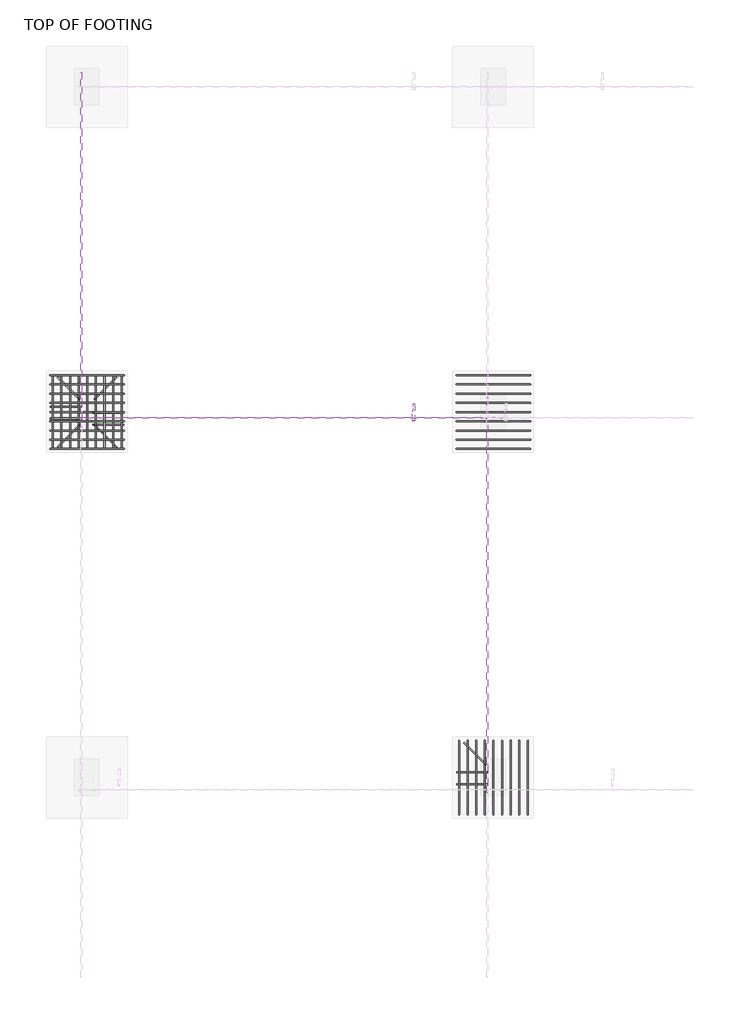
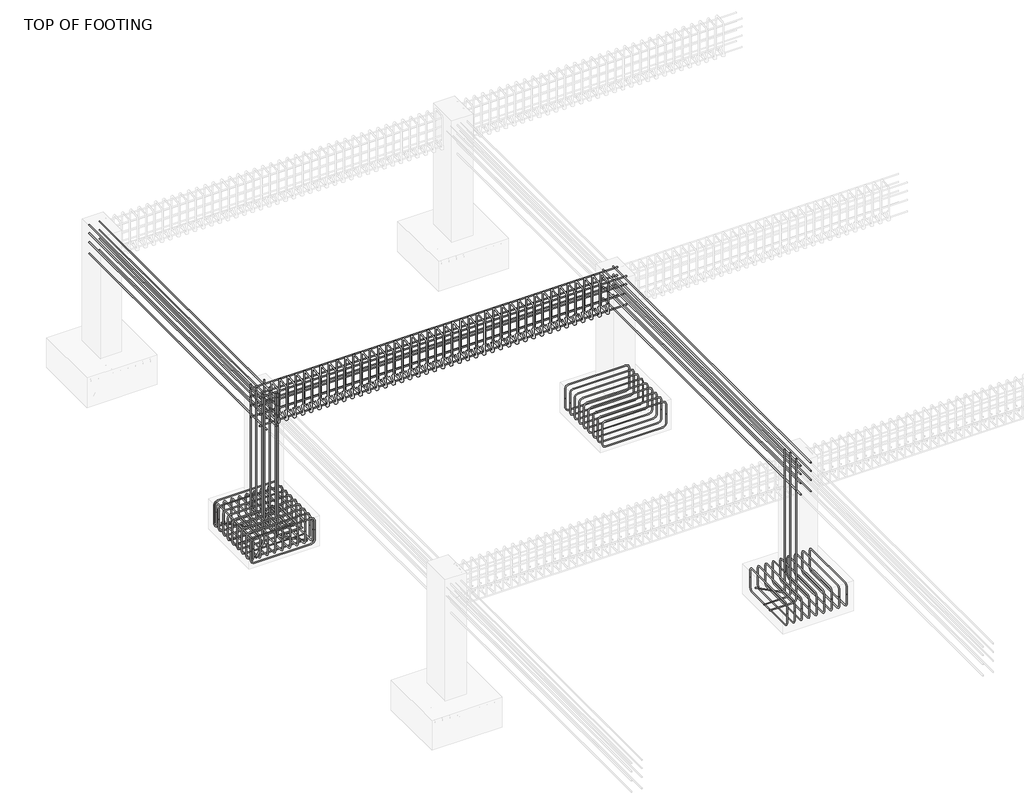
# One storey, part 5 of 13: 29 reinforcing bars.
"""IFC4 building model written with IfcOpenShell, lengths in millimetres."""

from ifc_helpers import new_model, si_unit, point, frame, origin, place, context, project, spatial, polyline, circle_curve, trimmed, segment, composite_curve, source, transform, mapped, element, save
from ifc_brep_helpers import swept_disk

model = new_model("IFC4")

# Units and contexts
model_context = context("Model", 3, world=origin())
ifc_project = project(units=[si_unit("LENGTHUNIT", "METRE", prefix="MILLI")], contexts=[model_context])

# Site, building, storey
site = spatial("IfcSite", under=ifc_project)
building = spatial("IfcBuilding", under=site)
storey = spatial("IfcBuildingStorey", under=building, Name="TOP OF FOOTING", Elevation=-1828.8)

# Reinforcing bars
placement = place(None, origin())
reinforcing_bar_shape = source(origin(), model_context, "Body", "SolidModel", [
    swept_disk(composite_curve([segment(polyline([(-12666.6498378, 12986.1851908, -2049.322685), (-12666.6498378, 12986.1851908, -2196.622685)]), True, "CONTINUOUS"), segment(trimmed(circle_curve(frame((-12712.9998378, 12986.1851908, -2196.622685), z_axis=(0.0, 1.0, 0.0), x_axis=(46.350000000000364, 0.0, 0.0)), 46.35), [point((-12666.6498378, 12986.1851908, -2196.622685))], [point((-12712.9998378, 12986.1851908, -2242.972685))], True, "CARTESIAN"), True, "CONTINUOUS"), segment(polyline([(-12712.9998378, 12986.1851908, -2242.972685), (-13527.5998378, 12986.1851908, -2242.972685)]), True, "CONTINUOUS"), segment(trimmed(circle_curve(frame((-13527.5998378, 12986.1851908, -2196.622685), z_axis=(0.0, 1.0, 0.0), x_axis=(0.0, 0.0, -46.350000000000364)), 46.35), [point((-13527.5998378, 12986.1851908, -2242.972685))], [point((-13573.9498378, 12986.1851908, -2196.622685))], True, "CARTESIAN"), True, "CONTINUOUS"), segment(polyline([(-13573.9498378, 12986.1851908, -2196.622685), (-13573.9498378, 12986.1851908, -2049.322685)]), True, "CONTINUOUS")], self_intersect=False), 6.35),
])
element("IfcReinforcingBar", 1, at=placement, inside=storey, context=model_context, shape_type="MappedRepresentation", body=[
    mapped(reinforcing_bar_shape, transform((0.0, 0.0, 0.0), x_axis=(1.0, 0.0, 0.0), y_axis=(0.0, 1.0, 0.0), z_axis=(0.0, 0.0, 1.0))),
    mapped(reinforcing_bar_shape, transform((0.0, -113.4125, 0.0), x_axis=(1.0, 0.0, 0.0), y_axis=(0.0, 1.0, 0.0), z_axis=(0.0, 0.0, 1.0))),
    mapped(reinforcing_bar_shape, transform((0.0, -226.825, 0.0), x_axis=(1.0, 0.0, 0.0), y_axis=(0.0, 1.0, 0.0), z_axis=(0.0, 0.0, 1.0))),
    mapped(reinforcing_bar_shape, transform((0.0, -340.2375, 0.0), x_axis=(1.0, 0.0, 0.0), y_axis=(0.0, 1.0, 0.0), z_axis=(0.0, 0.0, 1.0))),
    mapped(reinforcing_bar_shape, transform((0.0, -453.65, 0.0), x_axis=(1.0, 0.0, 0.0), y_axis=(0.0, 1.0, 0.0), z_axis=(0.0, 0.0, 1.0))),
    mapped(reinforcing_bar_shape, transform((0.0, -567.0625, 0.0), x_axis=(1.0, 0.0, 0.0), y_axis=(0.0, 1.0, 0.0), z_axis=(0.0, 0.0, 1.0))),
    mapped(reinforcing_bar_shape, transform((0.0, -680.475, 0.0), x_axis=(1.0, 0.0, 0.0), y_axis=(0.0, 1.0, 0.0), z_axis=(0.0, 0.0, 1.0))),
    mapped(reinforcing_bar_shape, transform((0.0, -793.8875, 0.0), x_axis=(1.0, 0.0, 0.0), y_axis=(0.0, 1.0, 0.0), z_axis=(0.0, 0.0, 1.0))),
    mapped(reinforcing_bar_shape, transform((0.0, -907.3, 0.0), x_axis=(1.0, 0.0, 0.0), y_axis=(0.0, 1.0, 0.0), z_axis=(0.0, 0.0, 1.0))),
])
reinforcing_bar_2_shape = source(origin(), model_context, "Body", "SolidModel", [
    swept_disk(composite_curve([segment(polyline([(-13573.9498378, 12986.1851908, -2051.3998363), (-13573.9498378, 12986.1851908, -1904.0998363)]), True, "CONTINUOUS"), segment(trimmed(circle_curve(frame((-13527.5998378, 12986.1851908, -1904.0998363), z_axis=(0.0, 1.0, 0.0), x_axis=(-46.350000000000364, 0.0, 0.0)), 46.35), [point((-13573.9498378, 12986.1851908, -1904.0998363))], [point((-13527.5998378, 12986.1851908, -1857.7498363))], True, "CARTESIAN"), True, "CONTINUOUS"), segment(polyline([(-13527.5998378, 12986.1851908, -1857.7498363), (-12712.9998378, 12986.1851908, -1857.7498363)]), True, "CONTINUOUS"), segment(trimmed(circle_curve(frame((-12712.9998378, 12986.1851908, -1904.0998363), z_axis=(0.0, 1.0, 0.0), x_axis=(0.0, 0.0, 46.350000000000136)), 46.35), [point((-12712.9998378, 12986.1851908, -1857.7498363))], [point((-12666.6498378, 12986.1851908, -1904.0998363))], True, "CARTESIAN"), True, "CONTINUOUS"), segment(polyline([(-12666.6498378, 12986.1851908, -1904.0998363), (-12666.6498378, 12986.1851908, -2051.3998363)]), True, "CONTINUOUS")], self_intersect=False), 6.35),
])
element("IfcReinforcingBar", 2, at=placement, inside=storey, context=model_context, shape_type="MappedRepresentation", body=[
    mapped(reinforcing_bar_2_shape, transform((0.0, 0.0, 0.0), x_axis=(1.0, 0.0, 0.0), y_axis=(0.0, 1.0, 0.0), z_axis=(0.0, 0.0, 1.0))),
    mapped(reinforcing_bar_2_shape, transform((0.0, -113.4125, 0.0), x_axis=(1.0, 0.0, 0.0), y_axis=(0.0, 1.0, 0.0), z_axis=(0.0, 0.0, 1.0))),
    mapped(reinforcing_bar_2_shape, transform((0.0, -226.825, 0.0), x_axis=(1.0, 0.0, 0.0), y_axis=(0.0, 1.0, 0.0), z_axis=(0.0, 0.0, 1.0))),
    mapped(reinforcing_bar_2_shape, transform((0.0, -340.2375, 0.0), x_axis=(1.0, 0.0, 0.0), y_axis=(0.0, 1.0, 0.0), z_axis=(0.0, 0.0, 1.0))),
    mapped(reinforcing_bar_2_shape, transform((0.0, -453.65, 0.0), x_axis=(1.0, 0.0, 0.0), y_axis=(0.0, 1.0, 0.0), z_axis=(0.0, 0.0, 1.0))),
    mapped(reinforcing_bar_2_shape, transform((0.0, -567.0625, 0.0), x_axis=(1.0, 0.0, 0.0), y_axis=(0.0, 1.0, 0.0), z_axis=(0.0, 0.0, 1.0))),
    mapped(reinforcing_bar_2_shape, transform((0.0, -680.475, 0.0), x_axis=(1.0, 0.0, 0.0), y_axis=(0.0, 1.0, 0.0), z_axis=(0.0, 0.0, 1.0))),
    mapped(reinforcing_bar_2_shape, transform((0.0, -793.8875, 0.0), x_axis=(1.0, 0.0, 0.0), y_axis=(0.0, 1.0, 0.0), z_axis=(0.0, 0.0, 1.0))),
    mapped(reinforcing_bar_2_shape, transform((0.0, -907.3, 0.0), x_axis=(1.0, 0.0, 0.0), y_axis=(0.0, 1.0, 0.0), z_axis=(0.0, 0.0, 1.0))),
])
reinforcing_bar_3_shape = source(origin(), model_context, "Body", "SolidModel", [
    swept_disk(composite_curve([segment(polyline([(-13542.4641345, 12986.1851908, -2025.081839), (-13542.4641345, 12986.1851908, -2172.381839)]), True, "CONTINUOUS"), segment(trimmed(circle_curve(frame((-13542.4641345, 12939.8351908, -2172.381839), z_axis=(-1.0, 0.0, 0.0), x_axis=(0.0, 46.350000000000364, 0.0)), 46.35), [point((-13542.4641345, 12986.1851908, -2172.381839))], [point((-13542.4641345, 12939.8351908, -2218.731839))], True, "CARTESIAN"), True, "CONTINUOUS"), segment(polyline([(-13542.4641345, 12939.8351908, -2218.731839), (-13542.4641345, 12125.2351908, -2218.731839)]), True, "CONTINUOUS"), segment(trimmed(circle_curve(frame((-13542.4641345, 12125.2351908, -2172.381839), z_axis=(-1.0, 0.0, 0.0), x_axis=(0.0, 0.0, -46.34999999999991)), 46.35), [point((-13542.4641345, 12125.2351908, -2218.731839))], [point((-13542.4641345, 12078.8851908, -2172.381839))], True, "CARTESIAN"), True, "CONTINUOUS"), segment(polyline([(-13542.4641345, 12078.8851908, -2172.381839), (-13542.4641345, 12078.8851908, -2025.081839)]), True, "CONTINUOUS")], self_intersect=False), 6.35),
])
element("IfcReinforcingBar", 3, at=placement, inside=storey, context=model_context, shape_type="MappedRepresentation", body=[
    mapped(reinforcing_bar_3_shape, transform((0.0, 0.0, 0.0), x_axis=(1.0, 0.0, 0.0), y_axis=(0.0, 1.0, 0.0), z_axis=(0.0, 0.0, 1.0))),
    mapped(reinforcing_bar_3_shape, transform((105.924033, 0.0, 0.0), x_axis=(1.0, 0.0, 0.0), y_axis=(0.0, 1.0, 0.0), z_axis=(0.0, 0.0, 1.0))),
    mapped(reinforcing_bar_3_shape, transform((211.8480661, 0.0, 0.0), x_axis=(1.0, 0.0, 0.0), y_axis=(0.0, 1.0, 0.0), z_axis=(0.0, 0.0, 1.0))),
    mapped(reinforcing_bar_3_shape, transform((317.7720991, 0.0, 0.0), x_axis=(1.0, 0.0, 0.0), y_axis=(0.0, 1.0, 0.0), z_axis=(0.0, 0.0, 1.0))),
    mapped(reinforcing_bar_3_shape, transform((423.6961321, 0.0, 0.0), x_axis=(1.0, 0.0, 0.0), y_axis=(0.0, 1.0, 0.0), z_axis=(0.0, 0.0, 1.0))),
    mapped(reinforcing_bar_3_shape, transform((529.6201652, 0.0, 0.0), x_axis=(1.0, 0.0, 0.0), y_axis=(0.0, 1.0, 0.0), z_axis=(0.0, 0.0, 1.0))),
    mapped(reinforcing_bar_3_shape, transform((635.5441982, 0.0, 0.0), x_axis=(1.0, 0.0, 0.0), y_axis=(0.0, 1.0, 0.0), z_axis=(0.0, 0.0, 1.0))),
    mapped(reinforcing_bar_3_shape, transform((741.4682312, 0.0, 0.0), x_axis=(1.0, 0.0, 0.0), y_axis=(0.0, 1.0, 0.0), z_axis=(0.0, 0.0, 1.0))),
    mapped(reinforcing_bar_3_shape, transform((847.3922643, 0.0, 0.0), x_axis=(1.0, 0.0, 0.0), y_axis=(0.0, 1.0, 0.0), z_axis=(0.0, 0.0, 1.0))),
])
reinforcing_bar_4_shape = source(origin(), model_context, "Body", "SolidModel", [
    swept_disk(composite_curve([segment(polyline([(-12695.0718702, 12986.1851908, -2069.0990329), (-12695.0718702, 12986.1851908, -1921.7990329)]), True, "CONTINUOUS"), segment(trimmed(circle_curve(frame((-12695.0718702, 12939.8351908, -1921.7990329), z_axis=(1.0, 0.0, 0.0), x_axis=(0.0, 46.350000000000364, 0.0)), 46.35), [point((-12695.0718702, 12986.1851908, -1921.7990329))], [point((-12695.0718702, 12939.8351908, -1875.4490329))], True, "CARTESIAN"), True, "CONTINUOUS"), segment(polyline([(-12695.0718702, 12939.8351908, -1875.4490329), (-12695.0718702, 12125.2351908, -1875.4490329)]), True, "CONTINUOUS"), segment(trimmed(circle_curve(frame((-12695.0718702, 12125.2351908, -1921.7990329), z_axis=(1.0, 0.0, 0.0), x_axis=(0.0, 0.0, 46.34999999999991)), 46.35), [point((-12695.0718702, 12125.2351908, -1875.4490329))], [point((-12695.0718702, 12078.8851908, -1921.7990329))], True, "CARTESIAN"), True, "CONTINUOUS"), segment(polyline([(-12695.0718702, 12078.8851908, -1921.7990329), (-12695.0718702, 12078.8851908, -2069.0990329)]), True, "CONTINUOUS")], self_intersect=False), 6.35),
])
element("IfcReinforcingBar", 4, at=placement, inside=storey, context=model_context, shape_type="MappedRepresentation", body=[
    mapped(reinforcing_bar_4_shape, transform((0.0, 0.0, 0.0), x_axis=(1.0, 0.0, 0.0), y_axis=(0.0, 1.0, 0.0), z_axis=(0.0, 0.0, 1.0))),
    mapped(reinforcing_bar_4_shape, transform((-105.924033, 0.0, 0.0), x_axis=(1.0, 0.0, 0.0), y_axis=(0.0, 1.0, 0.0), z_axis=(0.0, 0.0, 1.0))),
    mapped(reinforcing_bar_4_shape, transform((-211.8480661, 0.0, 0.0), x_axis=(1.0, 0.0, 0.0), y_axis=(0.0, 1.0, 0.0), z_axis=(0.0, 0.0, 1.0))),
    mapped(reinforcing_bar_4_shape, transform((-317.7720991, 0.0, 0.0), x_axis=(1.0, 0.0, 0.0), y_axis=(0.0, 1.0, 0.0), z_axis=(0.0, 0.0, 1.0))),
    mapped(reinforcing_bar_4_shape, transform((-423.6961321, 0.0, 0.0), x_axis=(1.0, 0.0, 0.0), y_axis=(0.0, 1.0, 0.0), z_axis=(0.0, 0.0, 1.0))),
    mapped(reinforcing_bar_4_shape, transform((-529.6201652, 0.0, 0.0), x_axis=(1.0, 0.0, 0.0), y_axis=(0.0, 1.0, 0.0), z_axis=(0.0, 0.0, 1.0))),
    mapped(reinforcing_bar_4_shape, transform((-635.5441982, 0.0, 0.0), x_axis=(1.0, 0.0, 0.0), y_axis=(0.0, 1.0, 0.0), z_axis=(0.0, 0.0, 1.0))),
    mapped(reinforcing_bar_4_shape, transform((-741.4682312, 0.0, 0.0), x_axis=(1.0, 0.0, 0.0), y_axis=(0.0, 1.0, 0.0), z_axis=(0.0, 0.0, 1.0))),
    mapped(reinforcing_bar_4_shape, transform((-847.3922643, 0.0, 0.0), x_axis=(1.0, 0.0, 0.0), y_axis=(0.0, 1.0, 0.0), z_axis=(0.0, 0.0, 1.0))),
])
reinforcing_bar_5_shape = source(origin(), model_context, "Body", "SolidModel", [
    swept_disk(composite_curve([segment(polyline([(-7666.6498378, 12986.1851908, -2049.322685), (-7666.6498378, 12986.1851908, -2196.622685)]), True, "CONTINUOUS"), segment(trimmed(circle_curve(frame((-7712.9998378, 12986.1851908, -2196.622685), z_axis=(0.0, 1.0, 0.0), x_axis=(46.350000000000364, 0.0, 0.0)), 46.35), [point((-7666.6498378, 12986.1851908, -2196.622685))], [point((-7712.9998378, 12986.1851908, -2242.972685))], True, "CARTESIAN"), True, "CONTINUOUS"), segment(polyline([(-7712.9998378, 12986.1851908, -2242.972685), (-8527.5998378, 12986.1851908, -2242.972685)]), True, "CONTINUOUS"), segment(trimmed(circle_curve(frame((-8527.5998378, 12986.1851908, -2196.622685), z_axis=(0.0, 1.0, 0.0), x_axis=(0.0, 0.0, -46.350000000000364)), 46.35), [point((-8527.5998378, 12986.1851908, -2242.972685))], [point((-8573.9498378, 12986.1851908, -2196.622685))], True, "CARTESIAN"), True, "CONTINUOUS"), segment(polyline([(-8573.9498378, 12986.1851908, -2196.622685), (-8573.9498378, 12986.1851908, -2049.322685)]), True, "CONTINUOUS")], self_intersect=False), 6.35),
])
element("IfcReinforcingBar", 5, at=placement, inside=storey, context=model_context, shape_type="MappedRepresentation", body=[
    mapped(reinforcing_bar_5_shape, transform((0.0, 0.0, 0.0), x_axis=(1.0, 0.0, 0.0), y_axis=(0.0, 1.0, 0.0), z_axis=(0.0, 0.0, 1.0))),
    mapped(reinforcing_bar_5_shape, transform((0.0, -113.4125, 0.0), x_axis=(1.0, 0.0, 0.0), y_axis=(0.0, 1.0, 0.0), z_axis=(0.0, 0.0, 1.0))),
    mapped(reinforcing_bar_5_shape, transform((0.0, -226.825, 0.0), x_axis=(1.0, 0.0, 0.0), y_axis=(0.0, 1.0, 0.0), z_axis=(0.0, 0.0, 1.0))),
    mapped(reinforcing_bar_5_shape, transform((0.0, -340.2375, 0.0), x_axis=(1.0, 0.0, 0.0), y_axis=(0.0, 1.0, 0.0), z_axis=(0.0, 0.0, 1.0))),
    mapped(reinforcing_bar_5_shape, transform((0.0, -453.65, 0.0), x_axis=(1.0, 0.0, 0.0), y_axis=(0.0, 1.0, 0.0), z_axis=(0.0, 0.0, 1.0))),
    mapped(reinforcing_bar_5_shape, transform((0.0, -567.0625, 0.0), x_axis=(1.0, 0.0, 0.0), y_axis=(0.0, 1.0, 0.0), z_axis=(0.0, 0.0, 1.0))),
    mapped(reinforcing_bar_5_shape, transform((0.0, -680.475, 0.0), x_axis=(1.0, 0.0, 0.0), y_axis=(0.0, 1.0, 0.0), z_axis=(0.0, 0.0, 1.0))),
    mapped(reinforcing_bar_5_shape, transform((0.0, -793.8875, 0.0), x_axis=(1.0, 0.0, 0.0), y_axis=(0.0, 1.0, 0.0), z_axis=(0.0, 0.0, 1.0))),
    mapped(reinforcing_bar_5_shape, transform((0.0, -907.3, 0.0), x_axis=(1.0, 0.0, 0.0), y_axis=(0.0, 1.0, 0.0), z_axis=(0.0, 0.0, 1.0))),
])
reinforcing_bar_6_shape = source(origin(), model_context, "Body", "SolidModel", [
    swept_disk(composite_curve([segment(polyline([(-8573.9498378, 12986.1851908, -2051.3998363), (-8573.9498378, 12986.1851908, -1904.0998363)]), True, "CONTINUOUS"), segment(trimmed(circle_curve(frame((-8527.5998378, 12986.1851908, -1904.0998363), z_axis=(0.0, 1.0, 0.0), x_axis=(-46.350000000000364, 0.0, 0.0)), 46.35), [point((-8573.9498378, 12986.1851908, -1904.0998363))], [point((-8527.5998378, 12986.1851908, -1857.7498363))], True, "CARTESIAN"), True, "CONTINUOUS"), segment(polyline([(-8527.5998378, 12986.1851908, -1857.7498363), (-7712.9998378, 12986.1851908, -1857.7498363)]), True, "CONTINUOUS"), segment(trimmed(circle_curve(frame((-7712.9998378, 12986.1851908, -1904.0998363), z_axis=(0.0, 1.0, 0.0), x_axis=(0.0, 0.0, 46.350000000000136)), 46.35), [point((-7712.9998378, 12986.1851908, -1857.7498363))], [point((-7666.6498378, 12986.1851908, -1904.0998363))], True, "CARTESIAN"), True, "CONTINUOUS"), segment(polyline([(-7666.6498378, 12986.1851908, -1904.0998363), (-7666.6498378, 12986.1851908, -2051.3998363)]), True, "CONTINUOUS")], self_intersect=False), 6.35),
])
element("IfcReinforcingBar", 6, at=placement, inside=storey, context=model_context, shape_type="MappedRepresentation", body=[
    mapped(reinforcing_bar_6_shape, transform((0.0, 0.0, 0.0), x_axis=(1.0, 0.0, 0.0), y_axis=(0.0, 1.0, 0.0), z_axis=(0.0, 0.0, 1.0))),
    mapped(reinforcing_bar_6_shape, transform((0.0, -113.4125, 0.0), x_axis=(1.0, 0.0, 0.0), y_axis=(0.0, 1.0, 0.0), z_axis=(0.0, 0.0, 1.0))),
    mapped(reinforcing_bar_6_shape, transform((0.0, -226.825, 0.0), x_axis=(1.0, 0.0, 0.0), y_axis=(0.0, 1.0, 0.0), z_axis=(0.0, 0.0, 1.0))),
    mapped(reinforcing_bar_6_shape, transform((0.0, -340.2375, 0.0), x_axis=(1.0, 0.0, 0.0), y_axis=(0.0, 1.0, 0.0), z_axis=(0.0, 0.0, 1.0))),
    mapped(reinforcing_bar_6_shape, transform((0.0, -453.65, 0.0), x_axis=(1.0, 0.0, 0.0), y_axis=(0.0, 1.0, 0.0), z_axis=(0.0, 0.0, 1.0))),
    mapped(reinforcing_bar_6_shape, transform((0.0, -567.0625, 0.0), x_axis=(1.0, 0.0, 0.0), y_axis=(0.0, 1.0, 0.0), z_axis=(0.0, 0.0, 1.0))),
    mapped(reinforcing_bar_6_shape, transform((0.0, -680.475, 0.0), x_axis=(1.0, 0.0, 0.0), y_axis=(0.0, 1.0, 0.0), z_axis=(0.0, 0.0, 1.0))),
    mapped(reinforcing_bar_6_shape, transform((0.0, -793.8875, 0.0), x_axis=(1.0, 0.0, 0.0), y_axis=(0.0, 1.0, 0.0), z_axis=(0.0, 0.0, 1.0))),
    mapped(reinforcing_bar_6_shape, transform((0.0, -907.3, 0.0), x_axis=(1.0, 0.0, 0.0), y_axis=(0.0, 1.0, 0.0), z_axis=(0.0, 0.0, 1.0))),
])
reinforcing_bar_7_shape = source(origin(), model_context, "Body", "SolidModel", [
    swept_disk(composite_curve([segment(polyline([(-8542.4641345, 8486.1851908, -2025.081839), (-8542.4641345, 8486.1851908, -2172.381839)]), True, "CONTINUOUS"), segment(trimmed(circle_curve(frame((-8542.4641345, 8439.8351908, -2172.381839), z_axis=(-1.0, 0.0, 0.0), x_axis=(0.0, 46.350000000000364, 0.0)), 46.35), [point((-8542.4641345, 8486.1851908, -2172.381839))], [point((-8542.4641345, 8439.8351908, -2218.731839))], True, "CARTESIAN"), True, "CONTINUOUS"), segment(polyline([(-8542.4641345, 8439.8351908, -2218.731839), (-8542.4641345, 7625.2351908, -2218.731839)]), True, "CONTINUOUS"), segment(trimmed(circle_curve(frame((-8542.4641345, 7625.2351908, -2172.381839), z_axis=(-1.0, 0.0, 0.0), x_axis=(0.0, 0.0, -46.34999999999991)), 46.35), [point((-8542.4641345, 7625.2351908, -2218.731839))], [point((-8542.4641345, 7578.8851908, -2172.381839))], True, "CARTESIAN"), True, "CONTINUOUS"), segment(polyline([(-8542.4641345, 7578.8851908, -2172.381839), (-8542.4641345, 7578.8851908, -2025.081839)]), True, "CONTINUOUS")], self_intersect=False), 6.35),
])
element("IfcReinforcingBar", 7, at=placement, inside=storey, context=model_context, shape_type="MappedRepresentation", body=[
    mapped(reinforcing_bar_7_shape, transform((0.0, 0.0, 0.0), x_axis=(1.0, 0.0, 0.0), y_axis=(0.0, 1.0, 0.0), z_axis=(0.0, 0.0, 1.0))),
    mapped(reinforcing_bar_7_shape, transform((105.924033, 0.0, 0.0), x_axis=(1.0, 0.0, 0.0), y_axis=(0.0, 1.0, 0.0), z_axis=(0.0, 0.0, 1.0))),
    mapped(reinforcing_bar_7_shape, transform((211.8480661, 0.0, 0.0), x_axis=(1.0, 0.0, 0.0), y_axis=(0.0, 1.0, 0.0), z_axis=(0.0, 0.0, 1.0))),
    mapped(reinforcing_bar_7_shape, transform((317.7720991, 0.0, 0.0), x_axis=(1.0, 0.0, 0.0), y_axis=(0.0, 1.0, 0.0), z_axis=(0.0, 0.0, 1.0))),
    mapped(reinforcing_bar_7_shape, transform((423.6961321, 0.0, 0.0), x_axis=(1.0, 0.0, 0.0), y_axis=(0.0, 1.0, 0.0), z_axis=(0.0, 0.0, 1.0))),
    mapped(reinforcing_bar_7_shape, transform((529.6201652, 0.0, 0.0), x_axis=(1.0, 0.0, 0.0), y_axis=(0.0, 1.0, 0.0), z_axis=(0.0, 0.0, 1.0))),
    mapped(reinforcing_bar_7_shape, transform((635.5441982, 0.0, 0.0), x_axis=(1.0, 0.0, 0.0), y_axis=(0.0, 1.0, 0.0), z_axis=(0.0, 0.0, 1.0))),
    mapped(reinforcing_bar_7_shape, transform((741.4682312, 0.0, 0.0), x_axis=(1.0, 0.0, 0.0), y_axis=(0.0, 1.0, 0.0), z_axis=(0.0, 0.0, 1.0))),
    mapped(reinforcing_bar_7_shape, transform((847.3922643, 0.0, 0.0), x_axis=(1.0, 0.0, 0.0), y_axis=(0.0, 1.0, 0.0), z_axis=(0.0, 0.0, 1.0))),
])
reinforcing_bar_8_shape = source(origin(), model_context, "Body", "SolidModel", [
    swept_disk(composite_curve([segment(polyline([(-7695.0718702, 8486.1851908, -2069.0990329), (-7695.0718702, 8486.1851908, -1921.7990329)]), True, "CONTINUOUS"), segment(trimmed(circle_curve(frame((-7695.0718702, 8439.8351908, -1921.7990329), z_axis=(1.0, 0.0, 0.0), x_axis=(0.0, 46.350000000000364, 0.0)), 46.35), [point((-7695.0718702, 8486.1851908, -1921.7990329))], [point((-7695.0718702, 8439.8351908, -1875.4490329))], True, "CARTESIAN"), True, "CONTINUOUS"), segment(polyline([(-7695.0718702, 8439.8351908, -1875.4490329), (-7695.0718702, 7625.2351908, -1875.4490329)]), True, "CONTINUOUS"), segment(trimmed(circle_curve(frame((-7695.0718702, 7625.2351908, -1921.7990329), z_axis=(1.0, 0.0, 0.0), x_axis=(0.0, 0.0, 46.34999999999991)), 46.35), [point((-7695.0718702, 7625.2351908, -1875.4490329))], [point((-7695.0718702, 7578.8851908, -1921.7990329))], True, "CARTESIAN"), True, "CONTINUOUS"), segment(polyline([(-7695.0718702, 7578.8851908, -1921.7990329), (-7695.0718702, 7578.8851908, -2069.0990329)]), True, "CONTINUOUS")], self_intersect=False), 6.35),
])
element("IfcReinforcingBar", 8, at=placement, inside=storey, context=model_context, shape_type="MappedRepresentation", body=[
    mapped(reinforcing_bar_8_shape, transform((0.0, 0.0, 0.0), x_axis=(1.0, 0.0, 0.0), y_axis=(0.0, 1.0, 0.0), z_axis=(0.0, 0.0, 1.0))),
    mapped(reinforcing_bar_8_shape, transform((-105.924033, 0.0, 0.0), x_axis=(1.0, 0.0, 0.0), y_axis=(0.0, 1.0, 0.0), z_axis=(0.0, 0.0, 1.0))),
    mapped(reinforcing_bar_8_shape, transform((-211.8480661, 0.0, 0.0), x_axis=(1.0, 0.0, 0.0), y_axis=(0.0, 1.0, 0.0), z_axis=(0.0, 0.0, 1.0))),
    mapped(reinforcing_bar_8_shape, transform((-317.7720991, 0.0, 0.0), x_axis=(1.0, 0.0, 0.0), y_axis=(0.0, 1.0, 0.0), z_axis=(0.0, 0.0, 1.0))),
    mapped(reinforcing_bar_8_shape, transform((-423.6961321, 0.0, 0.0), x_axis=(1.0, 0.0, 0.0), y_axis=(0.0, 1.0, 0.0), z_axis=(0.0, 0.0, 1.0))),
    mapped(reinforcing_bar_8_shape, transform((-529.6201652, 0.0, 0.0), x_axis=(1.0, 0.0, 0.0), y_axis=(0.0, 1.0, 0.0), z_axis=(0.0, 0.0, 1.0))),
    mapped(reinforcing_bar_8_shape, transform((-635.5441982, 0.0, 0.0), x_axis=(1.0, 0.0, 0.0), y_axis=(0.0, 1.0, 0.0), z_axis=(0.0, 0.0, 1.0))),
    mapped(reinforcing_bar_8_shape, transform((-741.4682312, 0.0, 0.0), x_axis=(1.0, 0.0, 0.0), y_axis=(0.0, 1.0, 0.0), z_axis=(0.0, 0.0, 1.0))),
    mapped(reinforcing_bar_8_shape, transform((-847.3922643, 0.0, 0.0), x_axis=(1.0, 0.0, 0.0), y_axis=(0.0, 1.0, 0.0), z_axis=(0.0, 0.0, 1.0))),
])
reinforcing_bar_9_shape = source(origin(), model_context, "Body", "SolidModel", [
    swept_disk(composite_curve([segment(polyline([(-13044.6810723, 12523.2621018, -40.0), (-13044.6810723, 12523.2621018, -2147.4714407)]), True, "CONTINUOUS"), segment(trimmed(circle_curve(frame((-12998.3310723, 12523.2621018, -2147.4714407), z_axis=(0.0, -1.0, 0.0), x_axis=(-46.350000000000364, 0.0, 0.0)), 46.35), [point((-13044.6810723, 12523.2621018, -2147.4714407))], [point((-12998.3310723, 12523.2621018, -2193.8214407))], True, "CARTESIAN"), True, "CONTINUOUS"), segment(polyline([(-12998.3310723, 12523.2621018, -2193.8214407), (-12667.4997506, 12523.2621018, -2193.8214407)]), True, "CONTINUOUS")], self_intersect=False), 6.35),
])
element("IfcReinforcingBar", 9, at=placement, inside=storey, context=model_context, shape_type="MappedRepresentation", body=[
    mapped(reinforcing_bar_9_shape, transform((0.0, 0.0, 0.0), x_axis=(1.0, 0.0, 0.0), y_axis=(0.0, 1.0, 0.0), z_axis=(0.0, 0.0, 1.0))),
    mapped(reinforcing_bar_9_shape, transform((0.0, -144.620853, 0.0), x_axis=(1.0, 0.0, 0.0), y_axis=(0.0, 1.0, 0.0), z_axis=(0.0, 0.0, 1.0))),
])
element("IfcReinforcingBar", 10, at=placement, inside=storey, context=model_context, shape_type="SolidModel", body=[
    swept_disk(composite_curve([segment(polyline([(-13024.6810723, 12696.1851908, -40.0), (-13024.6810723, 12696.1851908, -2147.4714407)]), True, "CONTINUOUS"), segment(trimmed(circle_curve(frame((-12991.906673, 12728.9595901, -2147.4714407), z_axis=(0.7071067811865476, -0.7071067811865475, 0.0), x_axis=(-32.77439930000037, -32.77439929999855, 0.0)), 46.35), [point((-13024.6810723, 12696.1851908, -2147.4714407))], [point((-12991.906673, 12728.9595901, -2193.8214407))], True, "CARTESIAN"), True, "CONTINUOUS"), segment(polyline([(-12991.906673, 12728.9595901, -2193.8214407), (-12757.973602, 12962.8926611, -2193.8214407)]), True, "CONTINUOUS")], self_intersect=False), 6.35),
])
element("IfcReinforcingBar", 11, at=placement, inside=storey, context=model_context, shape_type="SolidModel", body=[
    swept_disk(composite_curve([segment(polyline([(-13024.6810723, 12368.8851908, -40.0), (-13024.6810723, 12368.8851908, -2147.4714407)]), True, "CONTINUOUS"), segment(trimmed(circle_curve(frame((-12991.906673, 12336.1107915, -2147.4714407), z_axis=(-0.7071067811865542, -0.7071067811865408, 0.0), x_axis=(-32.77439930000037, 32.77439930000037, 0.0)), 46.35), [point((-13024.6810723, 12368.8851908, -2147.4714407))], [point((-12991.906673, 12336.1107915, -2193.8214407))], True, "CARTESIAN"), True, "CONTINUOUS"), segment(polyline([(-12991.906673, 12336.1107915, -2193.8214407), (-12757.973602, 12102.1777205, -2193.8214407)]), True, "CONTINUOUS")], self_intersect=False), 6.35),
])
element("IfcReinforcingBar", 12, at=placement, inside=storey, context=model_context, shape_type="SolidModel", body=[
    swept_disk(composite_curve([segment(polyline([(-13215.9186034, 12696.1851908, -40.0), (-13215.9186034, 12696.1851908, -2147.4714407)]), True, "CONTINUOUS"), segment(trimmed(circle_curve(frame((-13248.6930027, 12728.9595901, -2147.4714407), z_axis=(0.7071067811865679, 0.7071067811865271, 0.0), x_axis=(32.77439930000037, -32.77439929999855, 0.0)), 46.35), [point((-13215.9186034, 12696.1851908, -2147.4714407))], [point((-13248.6930027, 12728.9595901, -2193.8214407))], True, "CARTESIAN"), True, "CONTINUOUS"), segment(polyline([(-13248.6930027, 12728.9595901, -2193.8214407), (-13482.6260737, 12962.8926611, -2193.8214407)]), True, "CONTINUOUS")], self_intersect=False), 6.35),
])
element("IfcReinforcingBar", 13, at=placement, inside=storey, context=model_context, shape_type="SolidModel", body=[
    swept_disk(composite_curve([segment(polyline([(-13215.9186034, 12368.8851908, -40.0), (-13215.9186034, 12368.8851908, -2147.4714407)]), True, "CONTINUOUS"), segment(trimmed(circle_curve(frame((-13248.6930027, 12336.1107915, -2147.4714407), z_axis=(-0.7071067811865339, 0.7071067811865611, 0.0), x_axis=(32.77439930000037, 32.77439930000037, 0.0)), 46.35), [point((-13215.9186034, 12368.8851908, -2147.4714407))], [point((-13248.6930027, 12336.1107915, -2193.8214407))], True, "CARTESIAN"), True, "CONTINUOUS"), segment(polyline([(-13248.6930027, 12336.1107915, -2193.8214407), (-13482.6260737, 12102.1777205, -2193.8214407)]), True, "CONTINUOUS")], self_intersect=False), 6.35),
])
reinforcing_bar_10_shape = source(origin(), model_context, "Body", "SolidModel", [
    swept_disk(composite_curve([segment(polyline([(-13195.9186034, 12598.2621018, -40.0), (-13195.9186034, 12598.2621018, -2147.4714407)]), True, "CONTINUOUS"), segment(trimmed(circle_curve(frame((-13242.2686034, 12598.2621018, -2147.4714407), z_axis=(0.0, 1.0, 0.0), x_axis=(46.350000000000364, 0.0, 0.0)), 46.35), [point((-13195.9186034, 12598.2621018, -2147.4714407))], [point((-13242.2686034, 12598.2621018, -2193.8214407))], True, "CARTESIAN"), True, "CONTINUOUS"), segment(polyline([(-13242.2686034, 12598.2621018, -2193.8214407), (-13573.0999251, 12598.2621018, -2193.8214407)]), True, "CONTINUOUS")], self_intersect=False), 6.35),
])
element("IfcReinforcingBar", 14, at=placement, inside=storey, context=model_context, shape_type="MappedRepresentation", body=[
    mapped(reinforcing_bar_10_shape, transform((0.0, 0.0, 0.0), x_axis=(1.0, 0.0, 0.0), y_axis=(0.0, 1.0, 0.0), z_axis=(0.0, 0.0, 1.0))),
    mapped(reinforcing_bar_10_shape, transform((0.0, -144.620853, 0.0), x_axis=(1.0, 0.0, 0.0), y_axis=(0.0, 1.0, 0.0), z_axis=(0.0, 0.0, 1.0))),
])
element("IfcReinforcingBar", 15, at=placement, inside=storey, context=model_context, shape_type="SolidModel", body=[
    swept_disk(composite_curve([segment(polyline([(-8215.9186034, 8196.1851908, -40.0), (-8215.9186034, 8196.1851908, -2147.4714407)]), True, "CONTINUOUS"), segment(trimmed(circle_curve(frame((-8248.6930027, 8228.9595901, -2147.4714407), z_axis=(0.7071067811865679, 0.7071067811865271, 0.0), x_axis=(32.77439930000037, -32.77439929999855, 0.0)), 46.35), [point((-8215.9186034, 8196.1851908, -2147.4714407))], [point((-8248.6930027, 8228.9595901, -2193.8214407))], True, "CARTESIAN"), True, "CONTINUOUS"), segment(polyline([(-8248.6930027, 8228.9595901, -2193.8214407), (-8482.6260737, 8462.8926611, -2193.8214407)]), True, "CONTINUOUS")], self_intersect=False), 6.35),
])
reinforcing_bar_11_shape = source(origin(), model_context, "Body", "SolidModel", [
    swept_disk(composite_curve([segment(polyline([(-8195.9186034, 8098.2621018, -40.0), (-8195.9186034, 8098.2621018, -2147.4714407)]), True, "CONTINUOUS"), segment(trimmed(circle_curve(frame((-8242.2686034, 8098.2621018, -2147.4714407), z_axis=(0.0, 1.0, 0.0), x_axis=(46.350000000000364, 0.0, 0.0)), 46.35), [point((-8195.9186034, 8098.2621018, -2147.4714407))], [point((-8242.2686034, 8098.2621018, -2193.8214407))], True, "CARTESIAN"), True, "CONTINUOUS"), segment(polyline([(-8242.2686034, 8098.2621018, -2193.8214407), (-8573.0999251, 8098.2621018, -2193.8214407)]), True, "CONTINUOUS")], self_intersect=False), 6.35),
])
element("IfcReinforcingBar", 16, at=placement, inside=storey, context=model_context, shape_type="MappedRepresentation", body=[
    mapped(reinforcing_bar_11_shape, transform((0.0, 0.0, 0.0), x_axis=(1.0, 0.0, 0.0), y_axis=(0.0, 1.0, 0.0), z_axis=(0.0, 0.0, 1.0))),
    mapped(reinforcing_bar_11_shape, transform((0.0, -144.620853, 0.0), x_axis=(1.0, 0.0, 0.0), y_axis=(0.0, 1.0, 0.0), z_axis=(0.0, 0.0, 1.0))),
])
reinforcing_bar_12_shape = source(origin(), model_context, "Body", "SolidModel", [
    swept_disk(composite_curve([segment(polyline([(-8047.9242736, 12717.5351908, -87.6047527), (-8047.9242736, 7847.5351908, -87.6047527)]), True, "CONTINUOUS")], self_intersect=False), 6.35),
])
element("IfcReinforcingBar", 17, at=placement, inside=storey, context=model_context, shape_type="MappedRepresentation", body=[
    mapped(reinforcing_bar_12_shape, transform((0.0, 0.0, 0.0), x_axis=(1.0, 0.0, 0.0), y_axis=(0.0, 1.0, 0.0), z_axis=(0.0, 0.0, 1.0))),
    mapped(reinforcing_bar_12_shape, transform((-144.710816, 0.0, 0.0), x_axis=(1.0, 0.0, 0.0), y_axis=(0.0, 1.0, 0.0), z_axis=(0.0, 0.0, 1.0))),
])
reinforcing_bar_13_shape = source(origin(), model_context, "Body", "SolidModel", [
    swept_disk(composite_curve([segment(polyline([(-8047.9242736, 12717.5351908, -212.6047527), (-8047.9242736, 7847.5351908, -212.6047527)]), True, "CONTINUOUS")], self_intersect=False), 6.35),
])
element("IfcReinforcingBar", 18, at=placement, inside=storey, context=model_context, shape_type="MappedRepresentation", body=[
    mapped(reinforcing_bar_13_shape, transform((0.0, 0.0, 0.0), x_axis=(1.0, 0.0, 0.0), y_axis=(0.0, 1.0, 0.0), z_axis=(0.0, 0.0, 1.0))),
    mapped(reinforcing_bar_13_shape, transform((-144.710816, 0.0, 0.0), x_axis=(1.0, 0.0, 0.0), y_axis=(0.0, 1.0, 0.0), z_axis=(0.0, 0.0, 1.0))),
])
reinforcing_bar_14_shape = source(origin(), model_context, "Body", "SolidModel", [
    swept_disk(composite_curve([segment(polyline([(-8047.9242736, 12717.5351908, -517.6047527), (-8047.9242736, 7847.5351908, -517.6047527)]), True, "CONTINUOUS")], self_intersect=False), 6.35),
])
element("IfcReinforcingBar", 19, at=placement, inside=storey, context=model_context, shape_type="MappedRepresentation", body=[
    mapped(reinforcing_bar_14_shape, transform((0.0, 0.0, 0.0), x_axis=(1.0, 0.0, 0.0), y_axis=(0.0, 1.0, 0.0), z_axis=(0.0, 0.0, 1.0))),
    mapped(reinforcing_bar_14_shape, transform((-144.710816, 0.0, 0.0), x_axis=(1.0, 0.0, 0.0), y_axis=(0.0, 1.0, 0.0), z_axis=(0.0, 0.0, 1.0))),
])
reinforcing_bar_15_shape = source(origin(), model_context, "Body", "SolidModel", [
    swept_disk(composite_curve([segment(polyline([(-8047.9242736, 12717.5351908, -347.6047527), (-8047.9242736, 7847.5351908, -347.6047527)]), True, "CONTINUOUS")], self_intersect=False), 6.35),
])
element("IfcReinforcingBar", 20, at=placement, inside=storey, context=model_context, shape_type="MappedRepresentation", body=[
    mapped(reinforcing_bar_15_shape, transform((0.0, 0.0, 0.0), x_axis=(1.0, 0.0, 0.0), y_axis=(0.0, 1.0, 0.0), z_axis=(0.0, 0.0, 1.0))),
    mapped(reinforcing_bar_15_shape, transform((-144.710816, 0.0, 0.0), x_axis=(1.0, 0.0, 0.0), y_axis=(0.0, 1.0, 0.0), z_axis=(0.0, 0.0, 1.0))),
])
reinforcing_bar_16_shape = source(origin(), model_context, "Body", "SolidModel", [
    swept_disk(composite_curve([segment(polyline([(-13192.6754021, 12347.5351908, -87.6047527), (-13192.6754021, 16717.5351908, -87.6047527)]), True, "CONTINUOUS")], self_intersect=False), 6.35),
])
element("IfcReinforcingBar", 21, at=placement, inside=storey, context=model_context, shape_type="MappedRepresentation", body=[
    mapped(reinforcing_bar_16_shape, transform((0.0, 0.0, 0.0), x_axis=(1.0, 0.0, 0.0), y_axis=(0.0, 1.0, 0.0), z_axis=(0.0, 0.0, 1.0))),
    mapped(reinforcing_bar_16_shape, transform((144.710816, 0.0, 0.0), x_axis=(1.0, 0.0, 0.0), y_axis=(0.0, 1.0, 0.0), z_axis=(0.0, 0.0, 1.0))),
])
reinforcing_bar_17_shape = source(origin(), model_context, "Body", "SolidModel", [
    swept_disk(composite_curve([segment(polyline([(-13192.6754021, 12347.5351908, -212.6047527), (-13192.6754021, 16717.5351908, -212.6047527)]), True, "CONTINUOUS")], self_intersect=False), 6.35),
])
element("IfcReinforcingBar", 22, at=placement, inside=storey, context=model_context, shape_type="MappedRepresentation", body=[
    mapped(reinforcing_bar_17_shape, transform((0.0, 0.0, 0.0), x_axis=(1.0, 0.0, 0.0), y_axis=(0.0, 1.0, 0.0), z_axis=(0.0, 0.0, 1.0))),
    mapped(reinforcing_bar_17_shape, transform((144.710816, 0.0, 0.0), x_axis=(1.0, 0.0, 0.0), y_axis=(0.0, 1.0, 0.0), z_axis=(0.0, 0.0, 1.0))),
])
reinforcing_bar_18_shape = source(origin(), model_context, "Body", "SolidModel", [
    swept_disk(composite_curve([segment(polyline([(-13192.6754021, 12347.5351908, -517.6047527), (-13192.6754021, 16717.5351908, -517.6047527)]), True, "CONTINUOUS")], self_intersect=False), 6.35),
])
element("IfcReinforcingBar", 23, at=placement, inside=storey, context=model_context, shape_type="MappedRepresentation", body=[
    mapped(reinforcing_bar_18_shape, transform((0.0, 0.0, 0.0), x_axis=(1.0, 0.0, 0.0), y_axis=(0.0, 1.0, 0.0), z_axis=(0.0, 0.0, 1.0))),
    mapped(reinforcing_bar_18_shape, transform((144.710816, 0.0, 0.0), x_axis=(1.0, 0.0, 0.0), y_axis=(0.0, 1.0, 0.0), z_axis=(0.0, 0.0, 1.0))),
])
reinforcing_bar_19_shape = source(origin(), model_context, "Body", "SolidModel", [
    swept_disk(composite_curve([segment(polyline([(-13192.6754021, 12347.5351908, -347.6047527), (-13192.6754021, 16717.5351908, -347.6047527)]), True, "CONTINUOUS")], self_intersect=False), 6.35),
])
element("IfcReinforcingBar", 24, at=placement, inside=storey, context=model_context, shape_type="MappedRepresentation", body=[
    mapped(reinforcing_bar_19_shape, transform((0.0, 0.0, 0.0), x_axis=(1.0, 0.0, 0.0), y_axis=(0.0, 1.0, 0.0), z_axis=(0.0, 0.0, 1.0))),
    mapped(reinforcing_bar_19_shape, transform((144.710816, 0.0, 0.0), x_axis=(1.0, 0.0, 0.0), y_axis=(0.0, 1.0, 0.0), z_axis=(0.0, 0.0, 1.0))),
])
reinforcing_bar_20_shape = source(origin(), model_context, "Body", "SolidModel", [
    swept_disk(composite_curve([segment(polyline([(-12963.9498378, 12493.8109562, -444.3886395), (-12963.9498378, 12438.0673932, -500.1322024)]), True, "CONTINUOUS"), segment(trimmed(circle_curve(frame((-12963.9498378, 12460.2351908, -522.3), z_axis=(1.0, 0.0, 0.0), x_axis=(0.0, -22.167797599999176, 22.16779759999997)), 31.35), [point((-12963.9498378, 12438.0673932, -500.1322024))], [point((-12963.9498378, 12460.2351908, -553.65))], True, "CARTESIAN"), True, "CONTINUOUS"), segment(polyline([(-12963.9498378, 12460.2351908, -553.65), (-12963.9498378, 12604.8351908, -553.65)]), True, "CONTINUOUS"), segment(trimmed(circle_curve(frame((-12963.9498378, 12604.8351908, -522.3), z_axis=(1.0, 0.0, 0.0), x_axis=(0.0, 0.0, -31.350000000000023)), 31.35), [point((-12963.9498378, 12604.8351908, -553.65))], [point((-12963.9498378, 12636.1851908, -522.3))], True, "CARTESIAN"), True, "CONTINUOUS"), segment(polyline([(-12963.9498378, 12636.1851908, -522.3), (-12963.9498378, 12636.1851908, -77.7)]), True, "CONTINUOUS"), segment(trimmed(circle_curve(frame((-12965.8668659, 12604.8938581, -77.7), z_axis=(0.9981286353368323, -0.061149221750018364, 0.0), x_axis=(1.917028099998788, 31.291332700000567, 0.0)), 31.35), [point((-12963.9498378, 12636.1851908, -77.7))], [point((-12965.8668659, 12604.8938581, -46.35))], True, "CARTESIAN"), True, "CONTINUOUS"), segment(polyline([(-12965.8668659, 12604.8938581, -46.35), (-12974.7328097, 12460.1765235, -46.35)]), True, "CONTINUOUS"), segment(trimmed(circle_curve(frame((-12974.7328097, 12460.1765235, -77.7), z_axis=(0.9981286353368323, -0.061149221750018364, 0.0), x_axis=(0.0, 0.0, 31.35)), 31.35), [point((-12974.7328097, 12460.1765235, -46.35))], [point((-12976.6498378, 12428.8851908, -77.7))], True, "CARTESIAN"), True, "CONTINUOUS"), segment(polyline([(-12976.6498378, 12428.8851908, -77.7), (-12976.6498378, 12428.8851908, -522.3)]), True, "CONTINUOUS"), segment(trimmed(circle_curve(frame((-12976.6498378, 12460.2351908, -522.3), z_axis=(1.0, 0.0, 0.0), x_axis=(0.0, -31.350000000000364, 0.0)), 31.35), [point((-12976.6498378, 12428.8851908, -522.3))], [point((-12976.6498378, 12482.4029884, -544.4677976))], True, "CARTESIAN"), True, "CONTINUOUS"), segment(polyline([(-12976.6498378, 12482.4029884, -544.4677976), (-12976.6498378, 12538.1465513, -488.7242346)]), True, "CONTINUOUS")], self_intersect=False), 6.35),
])
element("IfcReinforcingBar", 25, at=placement, inside=storey, context=model_context, shape_type="MappedRepresentation", body=[
    mapped(reinforcing_bar_20_shape, transform((0.0, 0.0, 0.0), x_axis=(1.0, 0.0, 0.0), y_axis=(0.0, 1.0, 0.0), z_axis=(0.0, 0.0, 1.0))),
    mapped(reinforcing_bar_20_shape, transform((117.1825, 0.0, 0.0), x_axis=(1.0, 0.0, 0.0), y_axis=(0.0, 1.0, 0.0), z_axis=(0.0, 0.0, 1.0))),
    mapped(reinforcing_bar_20_shape, transform((234.365, 0.0, 0.0), x_axis=(1.0, 0.0, 0.0), y_axis=(0.0, 1.0, 0.0), z_axis=(0.0, 0.0, 1.0))),
    mapped(reinforcing_bar_20_shape, transform((351.5475, 0.0, 0.0), x_axis=(1.0, 0.0, 0.0), y_axis=(0.0, 1.0, 0.0), z_axis=(0.0, 0.0, 1.0))),
    mapped(reinforcing_bar_20_shape, transform((468.73, 0.0, 0.0), x_axis=(1.0, 0.0, 0.0), y_axis=(0.0, 1.0, 0.0), z_axis=(0.0, 0.0, 1.0))),
    mapped(reinforcing_bar_20_shape, transform((585.9125, 0.0, 0.0), x_axis=(1.0, 0.0, 0.0), y_axis=(0.0, 1.0, 0.0), z_axis=(0.0, 0.0, 1.0))),
    mapped(reinforcing_bar_20_shape, transform((703.095, 0.0, 0.0), x_axis=(1.0, 0.0, 0.0), y_axis=(0.0, 1.0, 0.0), z_axis=(0.0, 0.0, 1.0))),
    mapped(reinforcing_bar_20_shape, transform((820.2775, 0.0, 0.0), x_axis=(1.0, 0.0, 0.0), y_axis=(0.0, 1.0, 0.0), z_axis=(0.0, 0.0, 1.0))),
    mapped(reinforcing_bar_20_shape, transform((937.46, 0.0, 0.0), x_axis=(1.0, 0.0, 0.0), y_axis=(0.0, 1.0, 0.0), z_axis=(0.0, 0.0, 1.0))),
    mapped(reinforcing_bar_20_shape, transform((1054.6425, 0.0, 0.0), x_axis=(1.0, 0.0, 0.0), y_axis=(0.0, 1.0, 0.0), z_axis=(0.0, 0.0, 1.0))),
    mapped(reinforcing_bar_20_shape, transform((1171.825, 0.0, 0.0), x_axis=(1.0, 0.0, 0.0), y_axis=(0.0, 1.0, 0.0), z_axis=(0.0, 0.0, 1.0))),
    mapped(reinforcing_bar_20_shape, transform((1289.0075, 0.0, 0.0), x_axis=(1.0, 0.0, 0.0), y_axis=(0.0, 1.0, 0.0), z_axis=(0.0, 0.0, 1.0))),
    mapped(reinforcing_bar_20_shape, transform((1406.19, 0.0, 0.0), x_axis=(1.0, 0.0, 0.0), y_axis=(0.0, 1.0, 0.0), z_axis=(0.0, 0.0, 1.0))),
    mapped(reinforcing_bar_20_shape, transform((1523.3725, 0.0, 0.0), x_axis=(1.0, 0.0, 0.0), y_axis=(0.0, 1.0, 0.0), z_axis=(0.0, 0.0, 1.0))),
    mapped(reinforcing_bar_20_shape, transform((1640.555, 0.0, 0.0), x_axis=(1.0, 0.0, 0.0), y_axis=(0.0, 1.0, 0.0), z_axis=(0.0, 0.0, 1.0))),
    mapped(reinforcing_bar_20_shape, transform((1757.7375, 0.0, 0.0), x_axis=(1.0, 0.0, 0.0), y_axis=(0.0, 1.0, 0.0), z_axis=(0.0, 0.0, 1.0))),
    mapped(reinforcing_bar_20_shape, transform((1874.92, 0.0, 0.0), x_axis=(1.0, 0.0, 0.0), y_axis=(0.0, 1.0, 0.0), z_axis=(0.0, 0.0, 1.0))),
    mapped(reinforcing_bar_20_shape, transform((1992.1025, 0.0, 0.0), x_axis=(1.0, 0.0, 0.0), y_axis=(0.0, 1.0, 0.0), z_axis=(0.0, 0.0, 1.0))),
    mapped(reinforcing_bar_20_shape, transform((2109.285, 0.0, 0.0), x_axis=(1.0, 0.0, 0.0), y_axis=(0.0, 1.0, 0.0), z_axis=(0.0, 0.0, 1.0))),
    mapped(reinforcing_bar_20_shape, transform((2226.4675, 0.0, 0.0), x_axis=(1.0, 0.0, 0.0), y_axis=(0.0, 1.0, 0.0), z_axis=(0.0, 0.0, 1.0))),
    mapped(reinforcing_bar_20_shape, transform((2343.65, 0.0, 0.0), x_axis=(1.0, 0.0, 0.0), y_axis=(0.0, 1.0, 0.0), z_axis=(0.0, 0.0, 1.0))),
    mapped(reinforcing_bar_20_shape, transform((2460.8325, 0.0, 0.0), x_axis=(1.0, 0.0, 0.0), y_axis=(0.0, 1.0, 0.0), z_axis=(0.0, 0.0, 1.0))),
    mapped(reinforcing_bar_20_shape, transform((2578.015, 0.0, 0.0), x_axis=(1.0, 0.0, 0.0), y_axis=(0.0, 1.0, 0.0), z_axis=(0.0, 0.0, 1.0))),
    mapped(reinforcing_bar_20_shape, transform((2695.1975, 0.0, 0.0), x_axis=(1.0, 0.0, 0.0), y_axis=(0.0, 1.0, 0.0), z_axis=(0.0, 0.0, 1.0))),
    mapped(reinforcing_bar_20_shape, transform((2812.38, 0.0, 0.0), x_axis=(1.0, 0.0, 0.0), y_axis=(0.0, 1.0, 0.0), z_axis=(0.0, 0.0, 1.0))),
    mapped(reinforcing_bar_20_shape, transform((2929.5625, 0.0, 0.0), x_axis=(1.0, 0.0, 0.0), y_axis=(0.0, 1.0, 0.0), z_axis=(0.0, 0.0, 1.0))),
    mapped(reinforcing_bar_20_shape, transform((3046.745, 0.0, 0.0), x_axis=(1.0, 0.0, 0.0), y_axis=(0.0, 1.0, 0.0), z_axis=(0.0, 0.0, 1.0))),
    mapped(reinforcing_bar_20_shape, transform((3163.9275, 0.0, 0.0), x_axis=(1.0, 0.0, 0.0), y_axis=(0.0, 1.0, 0.0), z_axis=(0.0, 0.0, 1.0))),
    mapped(reinforcing_bar_20_shape, transform((3281.11, 0.0, 0.0), x_axis=(1.0, 0.0, 0.0), y_axis=(0.0, 1.0, 0.0), z_axis=(0.0, 0.0, 1.0))),
    mapped(reinforcing_bar_20_shape, transform((3398.2925, 0.0, 0.0), x_axis=(1.0, 0.0, 0.0), y_axis=(0.0, 1.0, 0.0), z_axis=(0.0, 0.0, 1.0))),
    mapped(reinforcing_bar_20_shape, transform((3515.475, 0.0, 0.0), x_axis=(1.0, 0.0, 0.0), y_axis=(0.0, 1.0, 0.0), z_axis=(0.0, 0.0, 1.0))),
    mapped(reinforcing_bar_20_shape, transform((3632.6575, 0.0, 0.0), x_axis=(1.0, 0.0, 0.0), y_axis=(0.0, 1.0, 0.0), z_axis=(0.0, 0.0, 1.0))),
    mapped(reinforcing_bar_20_shape, transform((3749.84, 0.0, 0.0), x_axis=(1.0, 0.0, 0.0), y_axis=(0.0, 1.0, 0.0), z_axis=(0.0, 0.0, 1.0))),
    mapped(reinforcing_bar_20_shape, transform((3867.0225, 0.0, 0.0), x_axis=(1.0, 0.0, 0.0), y_axis=(0.0, 1.0, 0.0), z_axis=(0.0, 0.0, 1.0))),
    mapped(reinforcing_bar_20_shape, transform((3984.205, 0.0, 0.0), x_axis=(1.0, 0.0, 0.0), y_axis=(0.0, 1.0, 0.0), z_axis=(0.0, 0.0, 1.0))),
    mapped(reinforcing_bar_20_shape, transform((4101.3875, 0.0, 0.0), x_axis=(1.0, 0.0, 0.0), y_axis=(0.0, 1.0, 0.0), z_axis=(0.0, 0.0, 1.0))),
    mapped(reinforcing_bar_20_shape, transform((4218.57, 0.0, 0.0), x_axis=(1.0, 0.0, 0.0), y_axis=(0.0, 1.0, 0.0), z_axis=(0.0, 0.0, 1.0))),
    mapped(reinforcing_bar_20_shape, transform((4335.7525, 0.0, 0.0), x_axis=(1.0, 0.0, 0.0), y_axis=(0.0, 1.0, 0.0), z_axis=(0.0, 0.0, 1.0))),
    mapped(reinforcing_bar_20_shape, transform((4452.935, 0.0, 0.0), x_axis=(1.0, 0.0, 0.0), y_axis=(0.0, 1.0, 0.0), z_axis=(0.0, 0.0, 1.0))),
    mapped(reinforcing_bar_20_shape, transform((4570.1175, 0.0, 0.0), x_axis=(1.0, 0.0, 0.0), y_axis=(0.0, 1.0, 0.0), z_axis=(0.0, 0.0, 1.0))),
    mapped(reinforcing_bar_20_shape, transform((4687.3, 0.0, 0.0), x_axis=(1.0, 0.0, 0.0), y_axis=(0.0, 1.0, 0.0), z_axis=(0.0, 0.0, 1.0))),
])
reinforcing_bar_21_shape = source(origin(), model_context, "Body", "SolidModel", [
    swept_disk(composite_curve([segment(polyline([(-13230.2998378, 12679.9107551, -87.6047527), (-8010.2998378, 12679.9107551, -87.6047527)]), True, "CONTINUOUS")], self_intersect=False), 6.35),
])
element("IfcReinforcingBar", 26, at=placement, inside=storey, context=model_context, shape_type="MappedRepresentation", body=[
    mapped(reinforcing_bar_21_shape, transform((0.0, 0.0, 0.0), x_axis=(1.0, 0.0, 0.0), y_axis=(0.0, 1.0, 0.0), z_axis=(0.0, 0.0, 1.0))),
    mapped(reinforcing_bar_21_shape, transform((0.0, -219.710816, 0.0), x_axis=(1.0, 0.0, 0.0), y_axis=(0.0, 1.0, 0.0), z_axis=(0.0, 0.0, 1.0))),
])
reinforcing_bar_22_shape = source(origin(), model_context, "Body", "SolidModel", [
    swept_disk(composite_curve([segment(polyline([(-13230.2998378, 12679.9107551, -212.6047527), (-8010.2998378, 12679.9107551, -212.6047527)]), True, "CONTINUOUS")], self_intersect=False), 6.35),
])
element("IfcReinforcingBar", 27, at=placement, inside=storey, context=model_context, shape_type="MappedRepresentation", body=[
    mapped(reinforcing_bar_22_shape, transform((0.0, 0.0, 0.0), x_axis=(1.0, 0.0, 0.0), y_axis=(0.0, 1.0, 0.0), z_axis=(0.0, 0.0, 1.0))),
    mapped(reinforcing_bar_22_shape, transform((0.0, -219.710816, 0.0), x_axis=(1.0, 0.0, 0.0), y_axis=(0.0, 1.0, 0.0), z_axis=(0.0, 0.0, 1.0))),
])
reinforcing_bar_23_shape = source(origin(), model_context, "Body", "SolidModel", [
    swept_disk(composite_curve([segment(polyline([(-13230.2998378, 12679.9107551, -517.6047527), (-8010.2998378, 12679.9107551, -517.6047527)]), True, "CONTINUOUS")], self_intersect=False), 6.35),
])
element("IfcReinforcingBar", 28, at=placement, inside=storey, context=model_context, shape_type="MappedRepresentation", body=[
    mapped(reinforcing_bar_23_shape, transform((0.0, 0.0, 0.0), x_axis=(1.0, 0.0, 0.0), y_axis=(0.0, 1.0, 0.0), z_axis=(0.0, 0.0, 1.0))),
    mapped(reinforcing_bar_23_shape, transform((0.0, -219.710816, 0.0), x_axis=(1.0, 0.0, 0.0), y_axis=(0.0, 1.0, 0.0), z_axis=(0.0, 0.0, 1.0))),
])
reinforcing_bar_24_shape = source(origin(), model_context, "Body", "SolidModel", [
    swept_disk(composite_curve([segment(polyline([(-13230.2998378, 12679.9107551, -347.6047527), (-8010.2998378, 12679.9107551, -347.6047527)]), True, "CONTINUOUS")], self_intersect=False), 6.35),
])
element("IfcReinforcingBar", 29, at=placement, inside=storey, context=model_context, shape_type="MappedRepresentation", body=[
    mapped(reinforcing_bar_24_shape, transform((0.0, 0.0, 0.0), x_axis=(1.0, 0.0, 0.0), y_axis=(0.0, 1.0, 0.0), z_axis=(0.0, 0.0, 1.0))),
    mapped(reinforcing_bar_24_shape, transform((0.0, -219.710816, 0.0), x_axis=(1.0, 0.0, 0.0), y_axis=(0.0, 1.0, 0.0), z_axis=(0.0, 0.0, 1.0))),
])

save(model, "model.ifc")

# Revit data of these elements
# Elements 1, 2, 3, 4, 5, 6, 7, 8, 9, 10, 11, 12, 13, 14, 15, 16, 17, 18, 19, 20, 21, 22, 23, 24, 25, 26, 27, 28, 29 (IfcReinforcingBar)
#   Phase Created = New Construction
